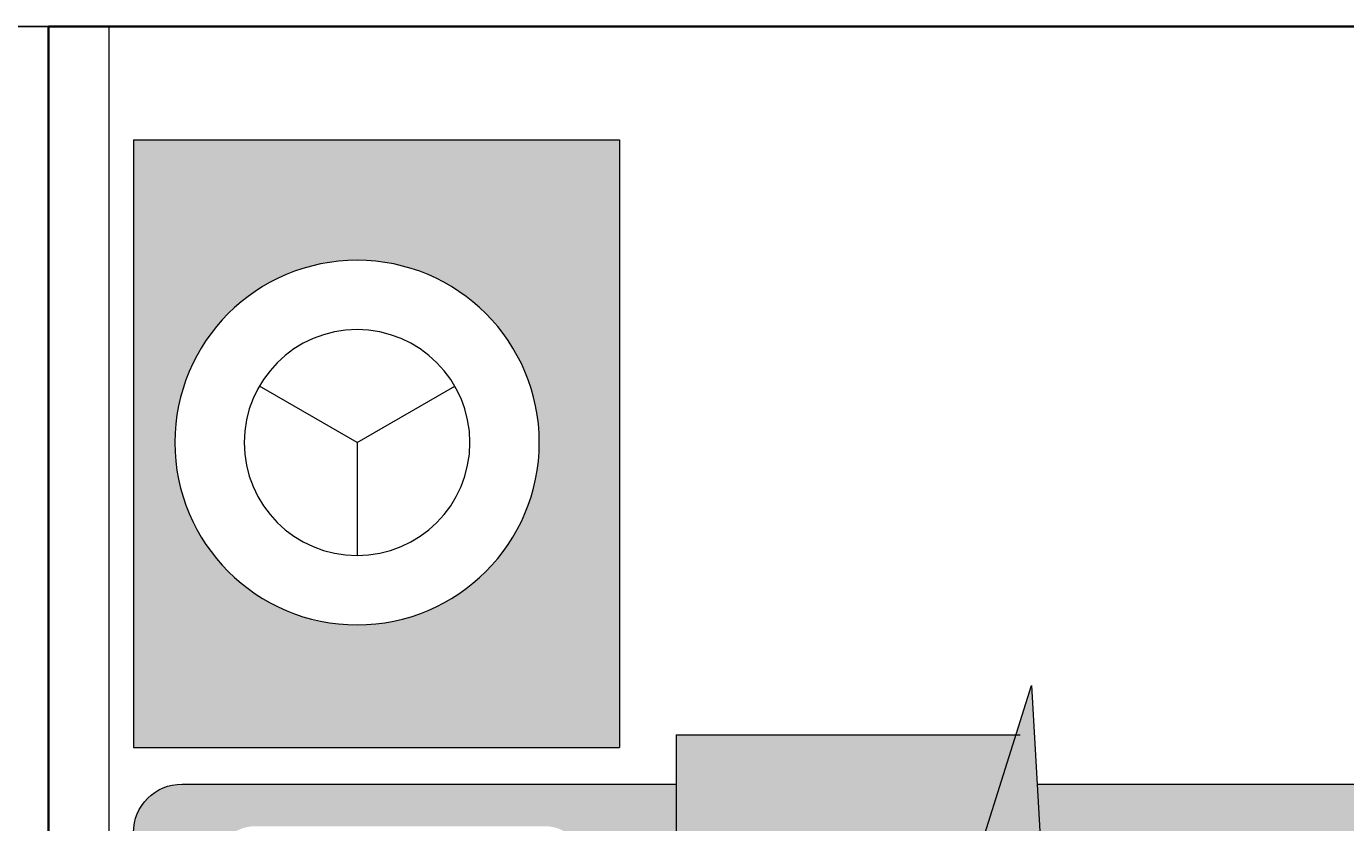
# Model space of a CAD drawing. Units: millimetres. Extents: x 27017497 to 27018854, y 7058029 to 7059154.
# Tile 85 of 91: x 27018319 to 27018362, y 7058555 to 7058581. Entities that reach past the tile are written whole.
import ezdxf

# ---------------------------------------------------------------- set-up
doc = ezdxf.new("R2010")
doc.units = ezdxf.units.MM
for name, color, linetype, lineweight in [('A-ANNO-DIMS', 2, 'Continuous', 18), ('A-FURN', 8, 'Continuous', 18), ('A-WALL', 7, 'Continuous', 35)]:
    doc.layers.add(name, color=color, linetype=linetype, lineweight=lineweight)
doc.layers.add('A-FURN-PATT', color=177, linetype='Continuous', lineweight=13, true_color=0x293189)
doc.styles.get("Standard").update_dxf_attribs({"font": 'arial.ttf'})
doc.dimstyles.get("Standard").update_dxf_attribs({"dimtxt": 0.18, "dimasz": 0.18, "dimexe": 0.18, "dimexo": 0.0625, "dimgap": 0.09, "dimtad": 0, "dimtih": 1, "dimtoh": 1, "dimdec": 4, "dimzin": 0, "dimdsep": 46, "dimtxsty": 'Standard', "dimcen": 0.09, "dimadec": 0, "dimazin": 0, "dimtfac": 1, "dimtdec": 4, "dimtofl": 0, "dimtmove": 0, "dimatfit": 3, "dimfxl": 1, "dimtolj": 1, "dimtzin": 0, "dimarcsym": 0})

# ---------------------------------------------------------------- blocks, each defined once
blk = doc.blocks.new('CAMMAT')
for p, q in [((1.2731, 0), (-1.2731, 0)), ((-1.2731, 0), (-1.2731, -0.05)), ((1.2731, -0.05), (-1.2731, -0.05)), ((-1.18, -0.07), (-1.18, -0.47)), ((-1.18, -0.07), (-0.68, -0.07)), ((-0.68, -0.07), (-0.68, -0.47)), ((-0.65, -0.11), (-0.65, -0.5169)), ((-0.931, -0.2541), (-0.9775, -0.1737)), ((-0.931, -0.2541), (-0.9775, -0.3346)), ((-0.931, -0.2541), (-0.8381, -0.2541)), ((-1.18, -0.47), (-0.68, -0.47)), ((-0.6904, -0.5169), (-0.6904, -0.8)), ((-0.6904, -0.5169), (0.6826, -0.5169)), ((0.0535, -0.5623), (-0.7312, -0.8093)), ((-0.65, -0.8139), (-0.65, -1.93))]:
    blk.add_line(p, q)
blk.add_lwpolyline([(-0.7312, -0.8093), (-0.5683, -0.8185), (-0.4451, -0.828), (-0.3552, -0.8406), (-0.2919, -0.8591), (-0.2489, -0.8862), (-0.2196, -0.9248), (-0.1975, -0.9777), (-0.1761, -1.0476)])
for radius in [0.15, 0.0929]:
    blk.add_circle((-0.931, -0.2541), radius)
blk.add_arc((-0.61, -0.11), 0.04, 90, 180)
blk = doc.blocks.new('*D48')
at = {"layer": 'A-ANNO-DIMS', "color": 0, "lineweight": -2, "transparency": 16777216}
for p, q in [((27018463.498, 7058622.912), (27017497.536, 7058622.912)), ((27017497.716, 7058622.732), (27017497.716, 7058357.753)), ((27017497.716, 7058092.41), (27017497.716, 7058357.389)), ((27018555.129, 7058092.23), (27017497.536, 7058092.23))]:
    blk.add_line(p, q, dxfattribs=at)
at = {"layer": 'A-ANNO-DIMS', "color": 0, "transparency": 16777216}
for points in [[(27017497.686, 7058622.732), (27017497.746, 7058622.732), (27017497.716, 7058622.912)], [(27017497.686, 7058092.41), (27017497.746, 7058092.41), (27017497.716, 7058092.23)]]:
    blk.add_solid(points, dxfattribs=at)
at = {"layer": 'Defpoints', "color": 0, "transparency": 16777216}
for p in [(27018463.561, 7058622.912), (27017497.716, 7058092.23), (27018555.192, 7058092.23)]:
    blk.add_point(p, dxfattribs=at)
at = {"layer": 'A-ANNO-DIMS', "color": 0, "transparency": 16777216, "insert": (27017497.716, 7058357.571), "char_height": 0.18, "attachment_point": 5}
blk.add_mtext('\\A1;530.7', dxfattribs=at)
blk = doc.blocks.new('*D50')
at = {"layer": 'A-ANNO-DIMS', "color": 0, "lineweight": -2, "transparency": 16777216}
for p, q in [((27018223.668, 7058580.912), (27018854.236, 7058580.912)), ((27018854.056, 7058580.732), (27018854.056, 7058511.344)), ((27018854.056, 7058441.592), (27018854.056, 7058510.98)), ((27018223.668, 7058441.412), (27018854.236, 7058441.412))]:
    blk.add_line(p, q, dxfattribs=at)
at = {"layer": 'A-ANNO-DIMS', "color": 0, "transparency": 16777216}
for points in [[(27018854.026, 7058580.732), (27018854.086, 7058580.732), (27018854.056, 7058580.912)], [(27018854.026, 7058441.592), (27018854.086, 7058441.592), (27018854.056, 7058441.412)]]:
    blk.add_solid(points, dxfattribs=at)
at = {"layer": 'Defpoints', "color": 0, "transparency": 16777216}
for p in [(27018223.606, 7058580.912), (27018223.606, 7058441.412), (27018854.056, 7058441.412)]:
    blk.add_point(p, dxfattribs=at)
at = {"layer": 'A-ANNO-DIMS', "color": 0, "transparency": 16777216, "insert": (27018854.056, 7058511.162), "char_height": 0.18, "attachment_point": 5}
blk.add_mtext('\\A1;139.5', dxfattribs=at)

msp = doc.modelspace()

# ---------------------------------------------------------------- hatches: boundary and pattern name
at = {"layer": 'A-FURN-PATT'}
h = msp.add_hatch(color=256, dxfattribs=at)
h.dxf.hatch_style = 1
h.paths.add_polyline_path([(27018398.067, 7058554.497, 0.414214), (27018396.474, 7058556.09), (27018352.018, 7058556.09), (27018352.202, 7058552.834), (27018352.581, 7058547.929), (27018353.082, 7058544.346), (27018353.818, 7058541.828), (27018354.899, 7058540.115), (27018356.437, 7058538.948), (27018358.543, 7058538.068), (27018361.329, 7058537.215), (27018358.524, 7058536.613), (27018356.284, 7058536.07), (27018354.381, 7058535.48), (27018352.588, 7058534.736), (27018350.68, 7058533.729), (27018348.431, 7058532.354), (27018345.612, 7058530.503), (27018341.998, 7058528.068), (27018345.612, 7058525.633), (27018348.431, 7058523.782), (27018350.68, 7058522.407), (27018352.588, 7058521.4), (27018354.381, 7058520.656), (27018356.284, 7058520.066), (27018358.524, 7058519.523), (27018361.329, 7058518.92), (27018358.543, 7058518.068), (27018356.437, 7058517.188), (27018354.899, 7058516.021), (27018353.818, 7058514.308), (27018353.082, 7058511.79), (27018352.581, 7058508.207), (27018352.28, 7058504.311), (27018396.474, 7058504.311, 0.414214), (27018398.067, 7058505.904)])
h.paths.add_polyline_path([(27018356.437, 7058538.948), (27018354.899, 7058540.115), (27018353.818, 7058541.828), (27018353.082, 7058544.346), (27018352.581, 7058547.929), (27018352.202, 7058552.834), (27018351.835, 7058559.322), (27018341.998, 7058528.068), (27018345.612, 7058530.503), (27018348.431, 7058532.354), (27018350.68, 7058533.729), (27018352.588, 7058534.736), (27018354.381, 7058535.48), (27018356.284, 7058536.07), (27018358.524, 7058536.613), (27018361.329, 7058537.215), (27018358.543, 7058538.068)])
h.paths.add_polyline_path([(27018358.543, 7058518.068), (27018361.329, 7058518.92), (27018358.524, 7058519.523), (27018356.284, 7058520.066), (27018354.381, 7058520.656), (27018352.588, 7058521.4), (27018350.68, 7058522.407), (27018348.431, 7058523.782), (27018345.612, 7058525.633), (27018341.998, 7058528.068), (27018351.835, 7058496.813), (27018352.202, 7058503.301), (27018352.581, 7058508.207), (27018353.082, 7058511.79), (27018353.818, 7058514.308), (27018354.899, 7058516.021), (27018356.437, 7058517.188)])
h.paths.add_polyline_path([(27018351.324, 7058557.699), (27018340.191, 7058557.699), (27018340.191, 7058503.014), (27018349.884, 7058503.014), (27018341.998, 7058528.068)])
h.paths.add_polyline_path([(27018340.191, 7058556.09), (27018323.983, 7058556.09, 0.414214), (27018322.39, 7058554.497), (27018322.39, 7058505.904, 0.414214), (27018323.983, 7058504.311), (27018340.191, 7058504.311)])
h.paths.add_polyline_path([(27018337.107, 7058532.051, -0.414214), (27018335.912, 7058530.856), (27018326.353, 7058530.856, -0.414214), (27018325.158, 7058532.051), (27018325.158, 7058553.51, -0.414214), (27018326.353, 7058554.705), (27018335.912, 7058554.705, -0.414214), (27018337.107, 7058553.51)], flags=0)
h.paths.add_polyline_path([(27018337.107, 7058527.914), (27018337.107, 7058506.454, -0.414214), (27018335.912, 7058505.259), (27018326.353, 7058505.259, -0.414214), (27018325.158, 7058506.454), (27018325.158, 7058527.914, -0.414214), (27018326.353, 7058529.109), (27018335.912, 7058529.109, -0.414214)], flags=0)
h.paths.add_polyline_path([(27018338.322, 7058577.2), (27018322.39, 7058577.2), (27018322.39, 7058557.285), (27018338.322, 7058557.285)])
h.paths.add_polyline_path([(27018323.748, 7058567.284, -1), (27018335.697, 7058567.284, -1)], flags=16)
h.paths.add_polyline_path([(27018326.023, 7058567.284, -1), (27018333.423, 7058567.284, -1)], flags=0)
h.paths.add_polyline_path([(27018338.322, 7058503.116), (27018322.39, 7058503.116), (27018322.39, 7058483.201), (27018338.322, 7058483.201)])
h.paths.add_polyline_path([(27018335.697, 7058493.391, -1), (27018323.748, 7058493.391, -1)], flags=16)
h.paths.add_polyline_path([(27018333.423, 7058493.391, -1), (27018326.023, 7058493.391, -1)], flags=0)
h.paths.add_polyline_path([(27018337.107, 7058527.914, 0.414214), (27018335.912, 7058529.109), (27018326.353, 7058529.109, 0.414214), (27018325.158, 7058527.914), (27018325.158, 7058506.454, 0.414214), (27018326.353, 7058505.259), (27018335.912, 7058505.259, 0.414214), (27018337.107, 7058506.454)], flags=16)
h.paths.add_polyline_path([(27018337.107, 7058553.51, 0.414214), (27018335.912, 7058554.705), (27018326.353, 7058554.705, 0.414214), (27018325.158, 7058553.51), (27018325.158, 7058532.051, 0.414214), (27018326.353, 7058530.856), (27018335.912, 7058530.856, 0.414214), (27018337.107, 7058532.051)], flags=16)

# ---------------------------------------------------------------- linework, layer by layer
at = {"layer": 'A-WALL'}
for p, q in [((27018319.606, 7058580.912), (27018319.606, 7058412.636)), ((27018729.106, 7058580.912), (27018319.606, 7058580.912))]:
    msp.add_line(p, q, dxfattribs=at)

# ---------------------------------------------------------------- block references
at = {"layer": 'A-FURN', "xscale": -39.82996475819422, "yscale": 39.82996475819422, "zscale": 39.82996475819422, "rotation": 90}
msp.add_blockref('CAMMAT', (27018319.602, 7058530.2), dxfattribs=at)

# ---------------------------------------------------------------- dimensions: what is measured, and where the dimension line sits
at = {"layer": 'A-ANNO-DIMS'}
for base, p1, p2, picture, middle in [((27017497.716, 7058092.23), (27018463.561, 7058622.912), (27018555.192, 7058092.23), '*D48', (27017497.716, 7058357.571)), ((27018854.056, 7058441.412), (27018223.606, 7058580.912), (27018223.606, 7058441.412), '*D50', (27018854.056, 7058511.162))]:
    dim = msp.add_linear_dim(base=base, p1=p1, p2=p2, angle=90, dimstyle='Standard', override={"dimdec": 1, "dimlfac": 1, "dimrnd": 0, "dimzin": 0, "dimdsep": 46, "dimlunit": 2}, dxfattribs=at)
    dim.commit()
    dim.dimension.update_dxf_attribs({"geometry": picture, "text_midpoint": middle})

doc.saveas('drawing.dxf')
